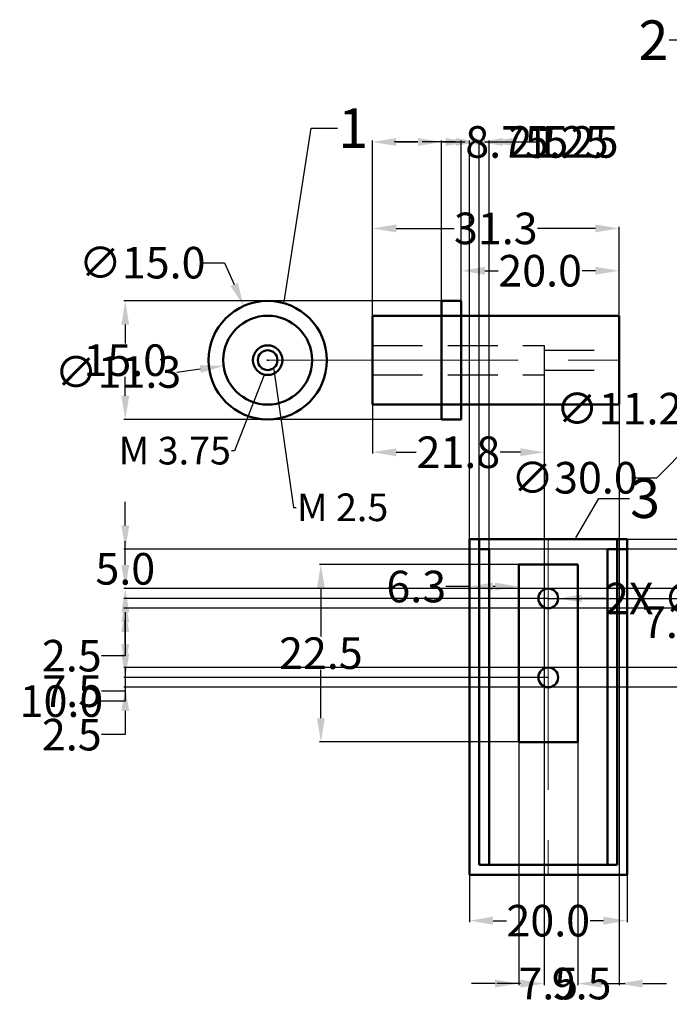
# Model space of a CAD drawing. Units: inches. Extents: x 0 to 231, y -13 to 111.
# Tile 1 of 3: x 0 to 83, y -13 to 111. Entities that reach past the tile are written whole.
import ezdxf
from ezdxf import colors
from ezdxf.entities.mleader import LeaderData, LeaderLine
from ezdxf.math import Vec2, Vec3

# ---------------------------------------------------------------- set-up
doc = ezdxf.new("R2010")
doc.units = ezdxf.units.IN
doc.header["$MEASUREMENT"] = 0
doc.linetypes.add('CENTER', pattern=[50.8, 31.75, -6.35, 6.35, -6.35])
doc.linetypes.add('HIDDEN', pattern=[9.525, 6.35, -3.175])
for name, color, linetype, lineweight in [('M-CNTR', 1, 'CENTER', 18), ('M-DIMS', 2, 'Continuous', 25), ('M-HIDN', 6, 'HIDDEN', 25), ('M-OUTL', 7, 'Continuous', 50), ('M-TEXT', 3, 'Continuous', 25)]:
    doc.layers.add(name, color=color, linetype=linetype, lineweight=lineweight)
doc.styles.get("Standard").update_dxf_attribs({"font": 'arial.ttf'})
doc.dimstyles.get("Standard").update_dxf_attribs({"dimtxt": 4, "dimasz": 3, "dimexe": 0.18, "dimexo": 0.0625, "dimgap": 0.09, "dimtad": 0, "dimtih": 1, "dimtoh": 1, "dimdec": 1, "dimzin": 0, "dimdsep": 46, "dimtxsty": 'Standard', "dimcen": 0.09, "dimadec": 0, "dimazin": 0, "dimtfac": 1, "dimtdec": 1, "dimtofl": 0, "dimtmove": 0, "dimatfit": 3, "dimfxl": 1, "dimtolj": 1, "dimtzin": 0, "dimarcsym": 0})

# ---------------------------------------------------------------- blocks, each defined once
blk = doc.blocks.new('*D1')
at = {"layer": 'Defpoints', "color": 0, "transparency": 16777216}
for p in [(76.44, 84.81), (45.19, 73.75), (76.44, 73.75)]:
    blk.add_point(p, dxfattribs=at)
at = {"layer": 'M-DIMS', "color": 0, "lineweight": -2, "transparency": 16777216}
for p, q in [((45.19, 73.81), (45.19, 84.99)), ((48.19, 84.81), (55.53, 84.81)), ((73.44, 84.81), (66.1, 84.81)), ((76.44, 73.81), (76.44, 84.99))]:
    blk.add_line(p, q, dxfattribs=at)
at = {"layer": 'M-DIMS', "color": 0, "transparency": 16777216}
for points in [[(48.19, 85.31), (48.19, 84.31), (45.19, 84.81)], [(73.44, 85.31), (73.44, 84.31), (76.44, 84.81)]]:
    blk.add_solid(points, dxfattribs=at)
at = {"layer": 'M-DIMS', "color": 0, "transparency": 16777216, "insert": (60.82, 84.81), "char_height": 4, "attachment_point": 5}
blk.add_mtext('\\A1;31.3', dxfattribs=at)
blk = doc.blocks.new('*D2')
at = {"layer": 'Defpoints', "color": 0, "transparency": 16777216}
for p in [(76.44, 79.45), (56.44, 74.79), (76.44, 74.79)]:
    blk.add_point(p, dxfattribs=at)
at = {"layer": 'M-DIMS', "color": 0, "lineweight": -2, "transparency": 16777216}
for p, q in [((56.44, 74.85), (56.44, 79.63)), ((59.44, 79.45), (61.13, 79.45)), ((73.44, 79.45), (71.76, 79.45)), ((76.44, 74.85), (76.44, 79.63))]:
    blk.add_line(p, q, dxfattribs=at)
at = {"layer": 'M-DIMS', "color": 0, "transparency": 16777216}
for points in [[(59.44, 79.95), (59.44, 78.95), (56.44, 79.45)], [(73.44, 79.95), (73.44, 78.95), (76.44, 79.45)]]:
    blk.add_solid(points, dxfattribs=at)
at = {"layer": 'M-DIMS', "color": 0, "transparency": 16777216, "insert": (66.44, 79.45), "char_height": 4, "attachment_point": 5}
blk.add_mtext('\\A1;20.0', dxfattribs=at)
blk = doc.blocks.new('*D3')
at = {"layer": 'Defpoints', "color": 0, "transparency": 16777216}
for p in [(45.19, 68.61), (66.94, 68.12), (45.19, 56.46)]:
    blk.add_point(p, dxfattribs=at)
at = {"layer": 'M-DIMS', "color": 0, "lineweight": -2, "transparency": 16777216}
for p, q in [((45.19, 68.55), (45.19, 56.28)), ((66.94, 68.06), (66.94, 56.28)), ((48.19, 56.46), (50.74, 56.46)), ((63.94, 56.46), (61.39, 56.46))]:
    blk.add_line(p, q, dxfattribs=at)
at = {"layer": 'M-DIMS', "color": 0, "transparency": 16777216}
for points in [[(48.19, 56.96), (48.19, 55.96), (45.19, 56.46)], [(63.94, 56.96), (63.94, 55.96), (66.94, 56.46)]]:
    blk.add_solid(points, dxfattribs=at)
at = {"layer": 'M-DIMS', "color": 0, "transparency": 16777216, "insert": (56.07, 56.46), "char_height": 4, "attachment_point": 5}
blk.add_mtext('\\A1;21.8', dxfattribs=at)
blk = doc.blocks.new('*D4')
at = {"layer": 'Defpoints', "color": 0, "transparency": 16777216}
for p in [(28.86, 74.98), (34.93, 61.26)]:
    blk.add_point(p, dxfattribs=at)
at = {"layer": 'M-DIMS', "color": 0, "lineweight": -2, "transparency": 16777216}
for p, q in [((23.43, 80.47), (26.43, 80.47)), ((26.43, 80.47), (27.65, 77.72)), ((31.8, 68.12), (31.98, 68.12)), ((31.89, 68.03), (31.89, 68.21))]:
    blk.add_line(p, q, dxfattribs=at)
at = {"layer": 'M-DIMS', "color": 0, "transparency": 16777216}
blk.add_solid([(28.1, 77.93), (27.19, 77.52), (28.86, 74.98)], dxfattribs=at)
at = {"layer": 'M-DIMS', "color": 0, "transparency": 16777216, "insert": (15.98, 80.47), "char_height": 4, "attachment_point": 5}
blk.add_mtext('\\A1;∅15.0', dxfattribs=at)
blk = doc.blocks.new('*D5')
at = {"layer": 'Defpoints', "color": 0, "transparency": 16777216}
for p in [(37.47, 68.85), (26.32, 67.4)]:
    blk.add_point(p, dxfattribs=at)
at = {"layer": 'M-DIMS', "color": 0, "lineweight": -2, "transparency": 16777216}
for p, q in [((31.8, 68.12), (31.98, 68.12)), ((31.89, 68.03), (31.89, 68.21)), ((20.37, 66.62), (23.34, 67.01))]:
    blk.add_line(p, q, dxfattribs=at)
at = {"layer": 'M-DIMS', "color": 0, "transparency": 16777216}
blk.add_solid([(23.28, 67.5), (23.41, 66.51), (26.32, 67.4)], dxfattribs=at)
at = {"layer": 'M-DIMS', "color": 0, "transparency": 16777216, "insert": (12.91, 66.62), "char_height": 4, "attachment_point": 5}
blk.add_mtext('\\A1;∅11.3', dxfattribs=at)
blk = doc.blocks.new('*D10')
at = {"layer": 'Defpoints', "color": 0, "transparency": 16777216}
for p in [(57.47, 2.94), (77.47, 2.94), (77.47, -2.87)]:
    blk.add_point(p, dxfattribs=at)
at = {"layer": 'M-DIMS', "color": 0, "lineweight": -2, "transparency": 16777216}
for p, q in [((57.47, 2.88), (57.47, -3.05)), ((77.47, 2.88), (77.47, -3.05)), ((60.47, -2.87), (62.16, -2.87)), ((74.47, -2.87), (72.78, -2.87))]:
    blk.add_line(p, q, dxfattribs=at)
at = {"layer": 'M-DIMS', "color": 0, "transparency": 16777216}
for points in [[(60.47, -2.37), (60.47, -3.37), (57.47, -2.87)], [(74.47, -2.37), (74.47, -3.37), (77.47, -2.87)]]:
    blk.add_solid(points, dxfattribs=at)
at = {"layer": 'M-DIMS', "color": 0, "transparency": 16777216, "insert": (67.47, -2.87), "char_height": 4, "attachment_point": 5}
blk.add_mtext('\\A1;20.0', dxfattribs=at)
blk = doc.blocks.new('*D11')
at = {"layer": 'Defpoints', "color": 0, "transparency": 16777216}
for p in [(65.59, 42.26), (38.64, 19.76), (65.59, 19.76)]:
    blk.add_point(p, dxfattribs=at)
at = {"layer": 'M-DIMS', "color": 0, "lineweight": -2, "transparency": 16777216}
for p, q in [((65.52, 42.26), (38.46, 42.26)), ((38.64, 39.26), (38.64, 33.14)), ((38.64, 22.76), (38.64, 28.88)), ((65.52, 19.76), (38.46, 19.76))]:
    blk.add_line(p, q, dxfattribs=at)
at = {"layer": 'M-DIMS', "color": 0, "transparency": 16777216}
for points in [[(38.14, 39.26), (39.14, 39.26), (38.64, 42.26)], [(38.14, 22.76), (39.14, 22.76), (38.64, 19.76)]]:
    blk.add_solid(points, dxfattribs=at)
at = {"layer": 'M-DIMS', "color": 0, "transparency": 16777216, "insert": (38.64, 31.01), "char_height": 4, "attachment_point": 5}
blk.add_mtext('\\A1;22.5', dxfattribs=at)
blk = doc.blocks.new('*D12')
at = {"layer": 'Defpoints', "color": 0, "transparency": 16777216}
for p in [(57.47, 45.44), (63.72, 42.26), (57.47, 39.45)]:
    blk.add_point(p, dxfattribs=at)
at = {"layer": 'M-DIMS', "color": 0, "lineweight": -2, "transparency": 16777216}
for p, q in [((57.47, 45.38), (57.47, 39.27)), ((63.72, 42.2), (63.72, 39.27)), ((57.47, 39.45), (54.47, 39.45)), ((60.72, 39.45), (60.47, 39.45))]:
    blk.add_line(p, q, dxfattribs=at)
at = {"layer": 'M-DIMS', "color": 0, "transparency": 16777216}
for points in [[(60.47, 39.95), (60.47, 38.95), (57.47, 39.45)], [(60.72, 39.95), (60.72, 38.95), (63.72, 39.45)]]:
    blk.add_solid(points, dxfattribs=at)
at = {"layer": 'M-DIMS', "color": 0, "transparency": 16777216, "insert": (50.73, 39.45), "char_height": 4, "attachment_point": 5}
blk.add_mtext('\\A1;6.3', dxfattribs=at)
blk = doc.blocks.new('*D13')
at = {"layer": 'Defpoints', "color": 0, "transparency": 16777216}
for p in [(67.47, 45.44), (67.47, 37.94), (89.87, 37.94)]:
    blk.add_point(p, dxfattribs=at)
at = {"layer": 'M-DIMS', "color": 0, "lineweight": -2, "transparency": 16777216}
for p, q in [((67.53, 45.44), (90.05, 45.44)), ((89.87, 42.44), (89.87, 40.94)), ((67.53, 37.94), (90.05, 37.94)), ((89.87, 37.94), (89.87, 34.94)), ((89.87, 34.94), (86.87, 34.94))]:
    blk.add_line(p, q, dxfattribs=at)
at = {"layer": 'M-DIMS', "color": 0, "transparency": 16777216}
for points in [[(89.37, 42.44), (90.37, 42.44), (89.87, 45.44)], [(89.37, 40.94), (90.37, 40.94), (89.87, 37.94)]]:
    blk.add_solid(points, dxfattribs=at)
at = {"layer": 'M-DIMS', "color": 0, "transparency": 16777216, "insert": (83.14, 34.94), "char_height": 4, "attachment_point": 5}
blk.add_mtext('\\A1;7.5', dxfattribs=at)
blk = doc.blocks.new('*D30')
at = {"layer": 'Defpoints', "color": 0, "transparency": 16777216}
for p in [(53.94, 95.76), (53.94, 75.62), (45.19, 73.75)]:
    blk.add_point(p, dxfattribs=at)
at = {"layer": 'M-DIMS', "color": 0, "lineweight": -2, "transparency": 16777216}
for p, q in [((45.19, 73.81), (45.19, 95.94)), ((48.19, 95.76), (50.94, 95.76)), ((53.94, 75.68), (53.94, 95.94)), ((53.94, 95.76), (56.94, 95.76))]:
    blk.add_line(p, q, dxfattribs=at)
at = {"layer": 'M-DIMS', "color": 0, "transparency": 16777216}
for points in [[(48.19, 96.26), (48.19, 95.26), (45.19, 95.76)], [(50.94, 96.26), (50.94, 95.26), (53.94, 95.76)]]:
    blk.add_solid(points, dxfattribs=at)
at = {"layer": 'M-DIMS', "color": 0, "transparency": 16777216, "insert": (62.25, 95.76), "char_height": 4, "attachment_point": 5}
blk.add_mtext('\\A1;8.75', dxfattribs=at)
blk = doc.blocks.new('*D31')
at = {"layer": 'Defpoints', "color": 0, "transparency": 16777216}
for p in [(56.44, 95.76), (53.94, 75.62), (56.44, 75.62)]:
    blk.add_point(p, dxfattribs=at)
at = {"layer": 'M-DIMS', "color": 0, "lineweight": -2, "transparency": 16777216}
for p, q in [((50.94, 95.76), (47.94, 95.76)), ((53.94, 75.68), (53.94, 95.94)), ((56.44, 75.68), (56.44, 95.94)), ((59.44, 95.76), (62.44, 95.76))]:
    blk.add_line(p, q, dxfattribs=at)
at = {"layer": 'M-DIMS', "color": 0, "transparency": 16777216}
for points in [[(50.94, 96.26), (50.94, 95.26), (53.94, 95.76)], [(59.44, 96.26), (59.44, 95.26), (56.44, 95.76)]]:
    blk.add_solid(points, dxfattribs=at)
at = {"layer": 'M-DIMS', "color": 0, "transparency": 16777216, "insert": (66.22, 95.76), "char_height": 4, "attachment_point": 5}
blk.add_mtext('\\A1;2.5', dxfattribs=at)
blk = doc.blocks.new('*D32')
at = {"layer": 'Defpoints', "color": 0, "transparency": 16777216}
for p in [(53.94, 75.62), (13.84, 60.62), (53.94, 60.62)]:
    blk.add_point(p, dxfattribs=at)
at = {"layer": 'M-DIMS', "color": 0, "lineweight": -2, "transparency": 16777216}
for p, q in [((53.88, 75.62), (13.66, 75.62)), ((13.84, 72.62), (13.84, 70.25)), ((13.84, 63.62), (13.84, 65.99)), ((53.88, 60.62), (13.66, 60.62))]:
    blk.add_line(p, q, dxfattribs=at)
at = {"layer": 'M-DIMS', "color": 0, "transparency": 16777216}
for points in [[(13.34, 72.62), (14.34, 72.62), (13.84, 75.62)], [(13.34, 63.62), (14.34, 63.62), (13.84, 60.62)]]:
    blk.add_solid(points, dxfattribs=at)
at = {"layer": 'M-DIMS', "color": 0, "transparency": 16777216, "insert": (13.84, 68.12), "char_height": 4, "attachment_point": 5}
blk.add_mtext('\\A1;15.0', dxfattribs=at)
blk = doc.blocks.new('*D33')
at = {"layer": 'Defpoints', "color": 0, "transparency": 16777216}
for p in [(66.943018, 66.871248), (76.443018, 62.496248), (76.443018, -10.838839)]:
    blk.add_point(p, dxfattribs=at)
at = {"layer": 'M-DIMS', "color": 0, "lineweight": -2, "transparency": 16777216}
for p, q in [((66.943018, 66.808748), (66.943018, -11.018839)), ((76.443018, 62.433748), (76.443018, -11.018839)), ((63.943018, -10.838839), (60.943018, -10.838839)), ((79.443018, -10.838839), (82.443018, -10.838839))]:
    blk.add_line(p, q, dxfattribs=at)
at = {"layer": 'M-DIMS', "color": 0, "transparency": 16777216}
for points in [[(63.943018, -10.338839), (63.943018, -11.338839), (66.943018, -10.838839)], [(79.443018, -10.338839), (79.443018, -11.338839), (76.443018, -10.838839)]]:
    blk.add_solid(points, dxfattribs=at)
at = {"layer": 'M-DIMS', "color": 0, "transparency": 16777216, "insert": (71.693018, -10.838839), "char_height": 4, "attachment_point": 5}
blk.add_mtext('\\A1;9.5', dxfattribs=at)
blk = doc.blocks.new('*D37')
at = {"layer": 'Defpoints', "color": 0, "transparency": 16777216}
for p in [(67.470797, 37.942783), (13.844426, 27.942783), (67.470797, 27.942783)]:
    blk.add_point(p, dxfattribs=at)
at = {"layer": 'M-DIMS', "color": 0, "lineweight": -2, "transparency": 16777216}
for p, q in [((67.408297, 37.942783), (13.664426, 37.942783)), ((13.844426, 34.942783), (13.844426, 30.942783)), ((67.408297, 27.942783), (13.664426, 27.942783)), ((13.844426, 27.942783), (13.844426, 24.942783)), ((13.844426, 24.942783), (10.844426, 24.942783))]:
    blk.add_line(p, q, dxfattribs=at)
at = {"layer": 'M-DIMS', "color": 0, "transparency": 16777216}
for points in [[(13.344426, 34.942783), (14.344426, 34.942783), (13.844426, 37.942783)], [(13.344426, 30.942783), (14.344426, 30.942783), (13.844426, 27.942783)]]:
    blk.add_solid(points, dxfattribs=at)
at = {"layer": 'M-DIMS', "color": 0, "transparency": 16777216, "insert": (5.754426, 24.942783), "char_height": 4, "attachment_point": 5}
blk.add_mtext('\\A1;10.0', dxfattribs=at)
blk = doc.blocks.new('*D38')
at = {"layer": 'Defpoints', "color": 0, "transparency": 16777216}
for p in [(63.720797, 19.758719), (71.220797, 19.758719), (71.220797, -10.838839)]:
    blk.add_point(p, dxfattribs=at)
at = {"layer": 'M-DIMS', "color": 0, "lineweight": -2, "transparency": 16777216}
for p, q in [((63.720797, 19.696219), (63.720797, -11.018839)), ((71.220797, 19.696219), (71.220797, -11.018839)), ((60.720797, -10.838839), (57.720797, -10.838839)), ((74.220797, -10.838839), (77.220797, -10.838839))]:
    blk.add_line(p, q, dxfattribs=at)
at = {"layer": 'M-DIMS', "color": 0, "transparency": 16777216}
for points in [[(60.720797, -10.338839), (60.720797, -11.338839), (63.720797, -10.838839)], [(74.220797, -10.338839), (74.220797, -11.338839), (71.220797, -10.838839)]]:
    blk.add_solid(points, dxfattribs=at)
at = {"layer": 'M-DIMS', "color": 0, "transparency": 16777216, "insert": (67.470797, -10.838839), "char_height": 4, "attachment_point": 5}
blk.add_mtext('\\A1;7.5', dxfattribs=at)
blk = doc.blocks.new('*D39')
at = {"layer": 'Defpoints', "color": 0, "transparency": 16777216}
for p in [(58.72, 95.76), (57.47, 45.44), (58.72, 45.44)]:
    blk.add_point(p, dxfattribs=at)
at = {"layer": 'M-DIMS', "color": 0, "lineweight": -2, "transparency": 16777216}
for p, q in [((54.47, 95.76), (51.47, 95.76)), ((57.47, 45.51), (57.47, 95.94)), ((58.72, 45.51), (58.72, 95.94)), ((61.72, 95.76), (64.72, 95.76))]:
    blk.add_line(p, q, dxfattribs=at)
at = {"layer": 'M-DIMS', "color": 0, "transparency": 16777216}
for points in [[(54.47, 96.26), (54.47, 95.26), (57.47, 95.76)], [(61.72, 96.26), (61.72, 95.26), (58.72, 95.76)]]:
    blk.add_solid(points, dxfattribs=at)
at = {"layer": 'M-DIMS', "color": 0, "transparency": 16777216, "insert": (69.83, 95.76), "char_height": 4, "attachment_point": 5}
blk.add_mtext('\\A1;1.25', dxfattribs=at)
blk = doc.blocks.new('*D40')
at = {"layer": 'Defpoints', "color": 0, "transparency": 16777216}
for p in [(59.97, 95.76), (58.72, 44.19), (59.97, 44.19)]:
    blk.add_point(p, dxfattribs=at)
at = {"layer": 'M-DIMS', "color": 0, "lineweight": -2, "transparency": 16777216}
for p, q in [((55.72, 95.76), (52.72, 95.76)), ((58.72, 44.26), (58.72, 95.94)), ((59.97, 44.26), (59.97, 95.94)), ((62.97, 95.76), (65.97, 95.76))]:
    blk.add_line(p, q, dxfattribs=at)
at = {"layer": 'M-DIMS', "color": 0, "transparency": 16777216}
for points in [[(55.72, 96.26), (55.72, 95.26), (58.72, 95.76)], [(62.97, 96.26), (62.97, 95.26), (59.97, 95.76)]]:
    blk.add_solid(points, dxfattribs=at)
at = {"layer": 'M-DIMS', "color": 0, "transparency": 16777216, "insert": (71.08, 95.76), "char_height": 4, "attachment_point": 5}
blk.add_mtext('\\A1;1.25', dxfattribs=at)
blk = doc.blocks.new('*D41')
at = {"layer": 'Defpoints', "color": 0, "transparency": 16777216}
for p in [(115.946436, 44.192783), (13.844426, 39.192783), (115.946436, 39.192783)]:
    blk.add_point(p, dxfattribs=at)
at = {"layer": 'M-DIMS', "color": 0, "lineweight": -2, "transparency": 16777216}
for p, q in [((13.844426, 47.192783), (13.844426, 50.192783)), ((115.883936, 44.192783), (13.664426, 44.192783)), ((115.883936, 39.192783), (13.664426, 39.192783)), ((13.844426, 36.192783), (13.844426, 33.192783))]:
    blk.add_line(p, q, dxfattribs=at)
at = {"layer": 'M-DIMS', "color": 0, "transparency": 16777216}
for points in [[(13.344426, 47.192783), (14.344426, 47.192783), (13.844426, 44.192783)], [(13.344426, 36.192783), (14.344426, 36.192783), (13.844426, 39.192783)]]:
    blk.add_solid(points, dxfattribs=at)
at = {"layer": 'M-DIMS', "color": 0, "transparency": 16777216, "insert": (13.844426, 41.692783), "char_height": 4, "attachment_point": 5}
blk.add_mtext('\\A1;5.0', dxfattribs=at)
blk = doc.blocks.new('*D42')
at = {"layer": 'Defpoints', "color": 0, "transparency": 16777216}
for p in [(115.95, 39.19), (13.84, 36.69), (115.95, 36.69)]:
    blk.add_point(p, dxfattribs=at)
at = {"layer": 'M-DIMS', "color": 0, "lineweight": -2, "transparency": 16777216}
for p, q in [((13.84, 42.19), (13.84, 45.19)), ((115.88, 39.19), (13.66, 39.19)), ((115.88, 36.69), (13.66, 36.69)), ((13.84, 33.69), (13.84, 30.69)), ((13.84, 30.69), (10.84, 30.69))]:
    blk.add_line(p, q, dxfattribs=at)
at = {"layer": 'M-DIMS', "color": 0, "transparency": 16777216}
for points in [[(13.34, 42.19), (14.34, 42.19), (13.84, 39.19)], [(13.34, 33.69), (14.34, 33.69), (13.84, 36.69)]]:
    blk.add_solid(points, dxfattribs=at)
at = {"layer": 'M-DIMS', "color": 0, "transparency": 16777216, "insert": (7.06, 30.69), "char_height": 4, "attachment_point": 5}
blk.add_mtext('\\A1;2.5', dxfattribs=at)
blk = doc.blocks.new('*D43')
at = {"layer": 'Defpoints', "color": 0, "transparency": 16777216}
for p in [(115.95, 36.69), (13.84, 29.19), (115.95, 29.19)]:
    blk.add_point(p, dxfattribs=at)
at = {"layer": 'M-DIMS', "color": 0, "lineweight": -2, "transparency": 16777216}
for p, q in [((115.88, 36.69), (13.66, 36.69)), ((13.84, 33.69), (13.84, 32.19)), ((115.88, 29.19), (13.66, 29.19)), ((13.84, 29.19), (13.84, 26.19)), ((13.84, 26.19), (10.84, 26.19))]:
    blk.add_line(p, q, dxfattribs=at)
at = {"layer": 'M-DIMS', "color": 0, "transparency": 16777216}
for points in [[(13.34, 33.69), (14.34, 33.69), (13.84, 36.69)], [(13.34, 32.19), (14.34, 32.19), (13.84, 29.19)]]:
    blk.add_solid(points, dxfattribs=at)
at = {"layer": 'M-DIMS', "color": 0, "transparency": 16777216, "insert": (7.11, 26.19), "char_height": 4, "attachment_point": 5}
blk.add_mtext('\\A1;7.5', dxfattribs=at)
blk = doc.blocks.new('*D44')
at = {"layer": 'Defpoints', "color": 0, "transparency": 16777216}
for p in [(115.95, 29.19), (13.84, 26.69), (115.95, 26.69)]:
    blk.add_point(p, dxfattribs=at)
at = {"layer": 'M-DIMS', "color": 0, "lineweight": -2, "transparency": 16777216}
for p, q in [((13.84, 32.19), (13.84, 35.19)), ((115.88, 29.19), (13.66, 29.19)), ((115.88, 26.69), (13.66, 26.69)), ((13.84, 23.69), (13.84, 20.69)), ((13.84, 20.69), (10.84, 20.69))]:
    blk.add_line(p, q, dxfattribs=at)
at = {"layer": 'M-DIMS', "color": 0, "transparency": 16777216}
for points in [[(13.34, 32.19), (14.34, 32.19), (13.84, 29.19)], [(13.34, 23.69), (14.34, 23.69), (13.84, 26.69)]]:
    blk.add_solid(points, dxfattribs=at)
at = {"layer": 'M-DIMS', "color": 0, "transparency": 16777216, "insert": (7.06, 20.69), "char_height": 4, "attachment_point": 5}
blk.add_mtext('\\A1;2.5', dxfattribs=at)
blk = doc.blocks.new('*D51')
at = {"layer": 'Defpoints', "color": 0, "transparency": 16777216}
for p in [(108.79, 80.83), (87.6, 59.6)]:
    blk.add_point(p, dxfattribs=at)
at = {"layer": 'M-DIMS', "color": 0, "lineweight": -2, "transparency": 16777216}
for p, q in [((98.1, 70.21), (98.28, 70.21)), ((98.19, 70.12), (98.19, 70.3)), ((81.24, 53.23), (85.48, 57.47)), ((78.24, 53.23), (81.24, 53.23))]:
    blk.add_line(p, q, dxfattribs=at)
at = {"layer": 'M-DIMS', "color": 0, "transparency": 16777216}
blk.add_solid([(85.12, 57.83), (85.83, 57.12), (87.6, 59.6)], dxfattribs=at)
at = {"layer": 'M-DIMS', "color": 0, "transparency": 16777216, "insert": (70.78, 53.23), "char_height": 4, "attachment_point": 5}
blk.add_mtext('\\A1;∅30.0', dxfattribs=at)
blk = doc.blocks.new('*D52')
at = {"layer": 'Defpoints', "color": 0, "transparency": 16777216}
for p in [(102.17, 74.19), (94.22, 66.23)]:
    blk.add_point(p, dxfattribs=at)
at = {"layer": 'M-DIMS', "color": 0, "lineweight": -2, "transparency": 16777216}
for p, q in [((98.1, 70.21), (98.28, 70.21)), ((98.19, 70.12), (98.19, 70.3)), ((89.98, 61.98), (92.1, 64.11)), ((86.98, 61.98), (89.98, 61.98))]:
    blk.add_line(p, q, dxfattribs=at)
at = {"layer": 'M-DIMS', "color": 0, "transparency": 16777216}
blk.add_solid([(91.75, 64.46), (92.45, 63.75), (94.22, 66.23)], dxfattribs=at)
at = {"layer": 'M-DIMS', "color": 0, "transparency": 16777216, "insert": (77.95, 61.98), "char_height": 4, "attachment_point": 5}
blk.add_mtext('\\A1;∅11.25', dxfattribs=at)
blk = doc.blocks.new('*D54')
at = {"layer": 'Defpoints', "color": 0, "transparency": 16777216}
for p in [(66.22, 37.95), (68.72, 37.94)]:
    blk.add_point(p, dxfattribs=at)
at = {"layer": 'M-DIMS', "color": 0, "lineweight": -2, "transparency": 16777216}
for p, q in [((67.38, 37.94), (67.56, 37.94)), ((67.47, 37.85), (67.47, 38.03)), ((74.72, 37.93), (71.72, 37.93))]:
    blk.add_line(p, q, dxfattribs=at)
at = {"layer": 'M-DIMS', "color": 0, "transparency": 16777216}
blk.add_solid([(71.72, 38.43), (71.72, 37.43), (68.72, 37.94)], dxfattribs=at)
at = {"layer": 'M-DIMS', "color": 0, "transparency": 16777216, "insert": (84.87, 37.93), "char_height": 4, "attachment_point": 5}
blk.add_mtext('\\A1;2X ∅2.5', dxfattribs=at)

msp = doc.modelspace()

# ---------------------------------------------------------------- linework, layer by layer
at = {"layer": 'M-CNTR'}
for p, q in [((31.8944, 68.1212), (76.443, 68.1212)), ((67.4708, 45.4428), (67.4708, 2.9428))]:
    msp.add_line(p, q, dxfattribs=at)
at = {"layer": 'M-HIDN'}
for p, q in [((45.193, 69.9962), (66.943, 69.9962)), ((66.943, 69.9962), (66.943, 66.2462)), ((66.943, 69.3712), (76.443, 69.3712)), ((45.193, 66.2462), (66.943, 66.2462)), ((66.943, 66.8712), (76.443, 66.8712))]:
    msp.add_line(p, q, dxfattribs=at)
at = {"layer": 'M-OUTL'}
for p, q in [((53.943, 75.6212), (56.443, 75.6212)), ((53.943, 75.6212), (53.943, 60.6212)), ((56.443, 75.6212), (56.443, 60.6212)), ((45.193, 73.7462), (45.193, 62.4962)), ((45.193, 73.7462), (76.443, 73.7462)), ((76.443, 73.7462), (76.443, 62.4962)), ((45.193, 62.4962), (76.443, 62.4962)), ((53.943, 60.6212), (56.443, 60.6212)), ((57.4708, 2.9428), (57.4708, 45.4428)), ((57.4708, 45.4428), (77.4708, 45.4428)), ((58.7208, 4.1928), (58.7208, 45.4428)), ((76.2208, 45.4428), (76.2208, 4.1928)), ((77.4708, 45.4428), (77.4708, 2.9428)), ((58.7208, 44.1928), (59.9708, 44.1928)), ((59.9708, 4.1928), (59.9708, 44.1928)), ((74.9708, 44.1928), (74.9708, 4.1928)), ((74.9708, 44.1928), (77.4708, 44.1928)), ((63.7208, 19.7587), (63.7208, 42.2587)), ((63.7208, 42.2587), (71.2208, 42.2587)), ((71.2208, 19.7587), (71.2208, 42.2587)), ((63.7208, 19.7587), (71.2208, 19.7587)), ((76.2208, 4.1928), (58.7208, 4.1928)), ((77.4708, 2.9428), (57.4708, 2.9428))]:
    msp.add_line(p, q, dxfattribs=at)
for centre, radius in [((31.8944, 68.1212), 7.5), ((31.8944, 68.1212), 5.625), ((31.8944, 68.1212), 1.875), ((31.8944, 68.1212), 1.25), ((67.4708, 37.9428), 1.25), ((67.4708, 27.9428), 1.25)]:
    msp.add_circle(centre, radius, dxfattribs=at)

# ---------------------------------------------------------------- dimensions: what is measured, and where the dimension line sits
at = {"layer": 'M-DIMS'}
for base, p1, p2, override, picture, middle in [((53.943, 95.7603), (45.193, 73.7462), (53.943, 75.6212), {"dimdec": 2, "dimlfac": 1, "dimrnd": 0, "dimzin": 0, "dimdsep": 46, "dimlunit": 2}, '*D30', (62.2458, 95.7603)), ((56.443, 95.7603), (53.943, 75.6212), (56.443, 75.6212), {"dimdec": 1, "dimlfac": 1, "dimrnd": 0, "dimzin": 0, "dimdsep": 46, "dimlunit": 2}, '*D31', (66.2233, 95.7603)), ((58.7208, 95.7603), (57.4708, 45.4428), (58.7208, 45.4428), {"dimdec": 2, "dimlfac": 1, "dimrnd": 0, "dimzin": 0, "dimdsep": 46, "dimlunit": 2}, '*D39', (69.8326, 95.7603)), ((59.9708, 95.7603), (58.7208, 44.1928), (59.9708, 44.1928), {"dimdec": 2, "dimlfac": 1, "dimrnd": 0, "dimzin": 0, "dimdsep": 46, "dimlunit": 2}, '*D40', (71.0826, 95.7603)), ((76.4430175949, 84.8122777658), (45.1930175949, 73.7462484269), (76.4430175949, 73.7462484269), {"dimclrd": 0, "dimclre": 0, "dimclrt": 0}, '*D1', (60.8180175949, 84.8122777658)), ((76.443, 79.4465), (56.443, 74.7895), (76.443, 74.7895), {"dimclrd": 0, "dimclre": 0, "dimclrt": 0}, '*D2', (66.443, 79.4465)), ((45.1930175949, 56.4649527692), (66.9430175949, 68.1212484269), (45.1930175949, 68.6138063945), {"dimclrd": 0, "dimclre": 0, "dimclrt": 0}, '*D3', (56.0680175949, 56.4649527692)), ((76.443, -10.8388), (66.943, 66.8712), (76.443, 62.4962), {"dimdec": 1, "dimlfac": 1, "dimrnd": 0, "dimzin": 0, "dimdsep": 46, "dimlunit": 2}, '*D33', (71.693, -10.8388)), ((57.4707969346, 39.4502880566), (63.7207969346, 42.2587188842), (57.4707969346, 45.4427826383), {"dimclrd": 0, "dimclre": 0, "dimclrt": 0}, '*D12', (50.7286823371, 39.4502880566)), ((71.2208, -10.8388), (63.7208, 19.7587), (71.2208, 19.7587), {"dimdec": 1, "dimlfac": 1, "dimrnd": 0, "dimzin": 0, "dimdsep": 46, "dimlunit": 2}, '*D38', (67.4708, -10.8388)), ((77.4708, -2.8694), (57.4708, 2.9428), (77.4708, 2.9428), {"dimclrd": 0, "dimclre": 0, "dimclrt": 0}, '*D10', (67.4708, -2.8694))]:
    dim = msp.add_linear_dim(base=base, p1=p1, p2=p2, dimstyle='Standard', override=override, dxfattribs=at)
    dim.commit()
    dim.dimension.update_dxf_attribs({"geometry": picture, "text_midpoint": middle})
for p1, p2, picture, middle in [((34.9297, 61.2629), (28.8592, 74.9796), '*D4', (15.9767, 80.4663)), ((37.4723828275, 68.8472131209), (26.3164695501, 67.3952837329), '*D5', (12.9055713729, 66.6209213927))]:
    dim = msp.add_diameter_dim_2p(p1=p1, p2=p2, dimstyle='Standard', override={"dimclrd": 0, "dimclre": 0, "dimclrt": 0}, dxfattribs=at)
    dim.commit()
    dim.dimension.update_dxf_attribs({"geometry": picture, "text_midpoint": middle})
for p1, p2, override, picture, middle in [((108.7917, 80.8252), (87.5953, 59.5953), {"dimdec": 1, "dimlfac": 1, "dimrnd": 0, "dimzin": 0, "dimdsep": 46, "dimlunit": 2}, '*D51', (70.7821, 53.2263)), ((102.1676, 74.1911), (94.2194, 66.2294), {"dimdec": 2, "dimlfac": 1, "dimrnd": 0, "dimzin": 0, "dimdsep": 46, "dimlunit": 2}, '*D52', (77.9504, 61.9832))]:
    dim = msp.add_diameter_dim_2p(p1=p1, p2=p2, dimstyle='Standard', override=override, dxfattribs=at)
    dim.commit()
    dim.dimension.update_dxf_attribs({"geometry": picture, "text_midpoint": middle, "dimtype": 163})
for base, p1, p2, override, picture, middle in [((13.8444, 60.6212), (53.943, 75.6212), (53.943, 60.6212), {"dimdec": 1, "dimlfac": 1, "dimrnd": 0, "dimzin": 0, "dimdsep": 46, "dimlunit": 2}, '*D32', (13.8444, 68.1212)), ((13.8444, 39.1928), (115.9464, 44.1928), (115.9464, 39.1928), {"dimdec": 1, "dimlfac": 1, "dimrnd": 0, "dimzin": 0, "dimdsep": 46, "dimlunit": 2}, '*D41', (13.8444, 41.6928)), ((13.8444, 36.6928), (115.9464, 39.1928), (115.9464, 36.6928), {"dimdec": 1, "dimlfac": 1, "dimrnd": 0, "dimzin": 0, "dimdsep": 46, "dimlunit": 2}, '*D42', (7.0641, 30.6928)), ((89.8714, 37.9428), (67.4708, 45.4428), (67.4708, 37.9428), {"dimclrd": 0, "dimclre": 0, "dimclrt": 0}, '*D13', (83.1415, 34.9428)), ((38.635, 19.7587), (65.5874, 42.2587), (65.5874, 19.7587), {"dimclrd": 0, "dimclre": 0, "dimclrt": 0}, '*D11', (38.635, 31.0087)), ((13.8444, 27.9428), (67.4708, 37.9428), (67.4708, 27.9428), {"dimdec": 1, "dimlfac": 1, "dimrnd": 0, "dimzin": 0, "dimdsep": 46, "dimlunit": 2}, '*D37', (5.7544, 24.9428)), ((13.8444, 29.1928), (115.9464, 36.6928), (115.9464, 29.1928), {"dimdec": 1, "dimlfac": 1, "dimrnd": 0, "dimzin": 0, "dimdsep": 46, "dimlunit": 2}, '*D43', (7.1146, 26.1928)), ((13.8444, 26.6928), (115.9464, 29.1928), (115.9464, 26.6928), {"dimdec": 1, "dimlfac": 1, "dimrnd": 0, "dimzin": 0, "dimdsep": 46, "dimlunit": 2}, '*D44', (7.0641, 20.6928))]:
    dim = msp.add_linear_dim(base=base, p1=p1, p2=p2, angle=90, dimstyle='Standard', override=override, dxfattribs=at)
    dim.commit()
    dim.dimension.update_dxf_attribs({"geometry": picture, "text_midpoint": middle})
dim = msp.add_diameter_dim_2p(p1=(66.2208, 37.9456), p2=(68.7208, 37.94), text='2X <>', dimstyle='Standard', override={"dimdec": 1, "dimlfac": 1, "dimrnd": 0, "dimzin": 0, "dimdsep": 46, "dimlunit": 2}, dxfattribs=at)
dim.commit()
dim.dimension.update_dxf_attribs({"geometry": '*D54', "text_midpoint": (74.7208, 37.9266)})

# ---------------------------------------------------------------- leaders
at = {"layer": 'M-TEXT'}
ml = msp.add_multileader_mtext('Standard', dxfattribs=at)
ml.set_content('2', color=256)
ml.set_leader_properties()
ml.build(insert=Vec2(0, 0))
ml.multileader.update_dxf_attribs({"dogleg_length": 0.36, "arrow_head_size": 0.18})
ctx = ml.context
ctx.base_point, ctx.char_height, ctx.arrow_head_size, ctx.landing_gap_size, ctx.plane_origin = Vec3(79.2964, 108.6563), 5, 0.18, 0.09, Vec3(92.632, 84.1412)
ctx.text_align_type = 2
notes = []
notes.append((ctx, [(0, (1, 1, 0), (85.2943, 108.6563), (-1, 0), 2.5062, [(0, [(92.632, 84.1412)], 0, [])])]))
ctx.mtext.insert, ctx.mtext.alignment, ctx.mtext.flow_direction = Vec3(82.6981, 111.1563), 3, 5
ml = msp.add_multileader_mtext('Standard', dxfattribs=at)
ml.set_content('1', color=256)
ml.set_leader_properties()
ml.build(insert=Vec2(0, 0))
ml.multileader.update_dxf_attribs({"dogleg_length": 0.36, "arrow_head_size": 0.18})
ctx = ml.context
ctx.base_point, ctx.char_height, ctx.arrow_head_size, ctx.landing_gap_size, ctx.plane_origin = Vec3(40.7393, 97.5081), 5, 0.18, 0.09, Vec3(33.9746, 75.327)
notes.append((ctx, [(0, (1, 1, 0), (37.4138, 97.5081), (1, 0), 3.3256, [(0, [(33.9746, 75.327)], 0, [])])]))
ctx.mtext.insert, ctx.mtext.flow_direction = Vec3(40.8293, 100.0081), 5
ml = msp.add_multileader_mtext('Standard', dxfattribs=at)
ml.set_content('M 3.75', color=256)
ml.set_leader_properties()
ml.build(insert=Vec2(0, 0))
ml.multileader.update_dxf_attribs({"dogleg_length": 0.36, "arrow_head_size": 0.18})
ctx = ml.context
ctx.base_point, ctx.char_height, ctx.arrow_head_size, ctx.landing_gap_size, ctx.plane_origin = Vec3(12.7522, 56.6302), 3.5, 0.18, 0.09, Vec3(31.4583, 66.2977)
ctx.text_align_type = 2
notes.append((ctx, [(0, (1, 1, 0), (27.6814, 56.6302), (-1, 0), 0.36, [(0, [(31.4583, 66.2977)], 0, [])])]))
ctx.mtext.insert, ctx.mtext.alignment, ctx.mtext.flow_direction = Vec3(27.2314, 58.4112), 3, 5
ml = msp.add_multileader_mtext('Standard', dxfattribs=at)
ml.set_content('M 2.5', color=256)
ml.set_leader_properties()
ml.build(insert=Vec2(0, 0))
ml.multileader.update_dxf_attribs({"dogleg_length": 0.36, "arrow_head_size": 0.18})
ctx = ml.context
ctx.base_point, ctx.char_height, ctx.arrow_head_size, ctx.landing_gap_size, ctx.plane_origin = Vec3(35.5217, 49.4524), 3.5, 0.18, 0.09, Vec3(32.6305, 67.111)
notes.append((ctx, [(0, (1, 1, 0), (35.1617, 49.4524), (1, 0), 0.36, [(0, [(32.6305, 67.111)], 0, [])])]))
ctx.mtext.insert, ctx.mtext.flow_direction = Vec3(35.6117, 51.2322), 5
ml = msp.add_multileader_mtext('Standard', dxfattribs=at)
ml.set_content('3', color=256)
ml.set_leader_properties()
ml.build(insert=Vec2(0, 0))
ml.multileader.update_dxf_attribs({"dogleg_length": 0.36, "arrow_head_size": 0.18})
ctx = ml.context
ctx.base_point, ctx.char_height, ctx.arrow_head_size, ctx.landing_gap_size, ctx.plane_origin = Vec3(77.7603, 50.5903), 5, 0.18, 0.09, Vec3(70.8946, 45.4428)
notes.append((ctx, [(0, (1, 1, 0), (73.8665, 50.5903), (1, 0), 3.8938, [(0, [(70.8946, 45.4428)], 0, [])])]))
ctx.mtext.insert, ctx.mtext.flow_direction = Vec3(77.8503, 53.1346), 5
for ctx, leaders in notes:
    for number, flags, end, landing, length, lines in leaders:
        leader = LeaderData()
        leader.index, (leader.has_last_leader_line, leader.has_dogleg_vector, leader.attachment_direction) = number, flags
        leader.last_leader_point, leader.dogleg_vector, leader.dogleg_length = Vec3(end), Vec3(landing), length
        for number, points, colour, breaks in lines:
            line = LeaderLine()
            line.index, line.vertices, line.color, line.breaks = number, Vec3.list(points), colors.encode_raw_color(colour), breaks
            leader.lines.append(line)
        ctx.leaders.append(leader)

doc.saveas('drawing.dxf')
